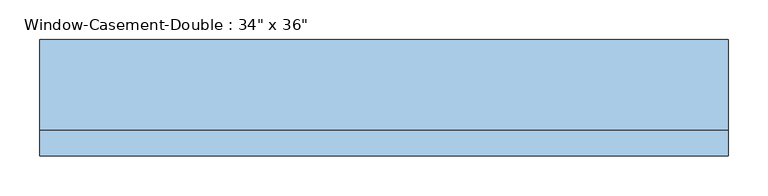
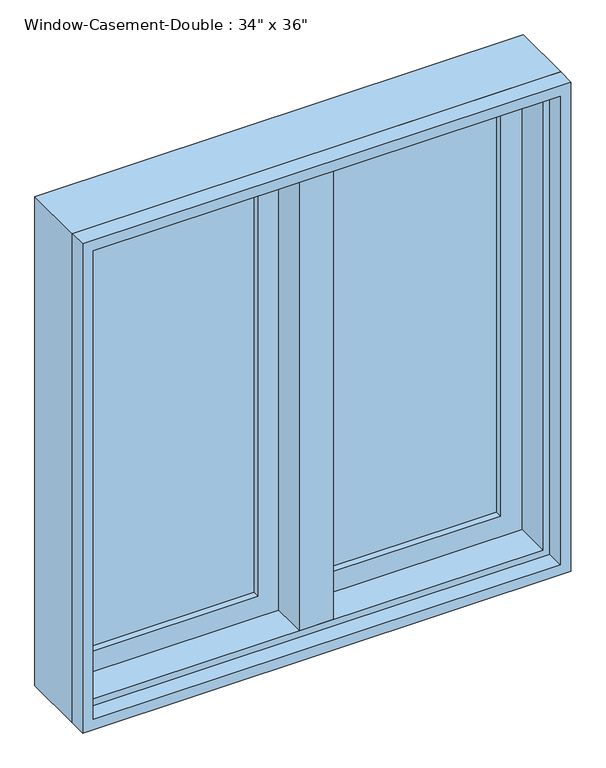
"""IFC4 building model written with IfcOpenShell, lengths in millimetres: window geometry."""

from ifc_helpers import new_model, si_unit, frame, origin, place, context, project, spatial, polyline, outline, extrude, faceted_brep, source, transform, mapped, element, save


def window_0d9958e7(model_context):
    return source(origin(), model_context, "Body", "SolidModel", [
        faceted_brep([(9.525, 82.55, 1816.1), (-9.525, 82.55, 1816.1), (-9.525, 31.75, 1816.1), (9.525, 31.75, 1816.1), (9.525, 82.55, 927.1), (9.525, 31.75, 927.1), (-9.525, 31.75, 927.1), (-9.525, 82.55, 927.1), (-9.525, 31.75, 946.15), (-9.525, 31.75, 1797.05), (-30.1625, 31.75, 946.15), (-30.1625, 31.75, 1797.05), (-30.1625, -31.75, 946.15), (-30.1625, -31.75, 1797.05), (30.1625, -31.75, 946.15), (30.1625, -31.75, 1797.05), (30.1625, 31.75, 946.15), (30.1625, 31.75, 1797.05), (9.525, 31.75, 946.15), (9.525, 31.75, 1797.05)], [[[0, 1, 2, 3]], [[4, 5, 6, 7]], [[1, 0, 4, 7]], [[2, 1, 7, 6, 8, 9]], [[9, 8, 10, 11]], [[11, 10, 12, 13]], [[13, 12, 14, 15]], [[15, 14, 16, 17]], [[17, 16, 18, 19]], [[0, 3, 19, 18, 5, 4]], [[18, 8, 6, 5]], [[9, 19, 3, 2]], [[8, 18, 16, 14, 12, 10]], [[19, 9, 11, 13, 15, 17]]]),
        extrude(outline(polyline([(-66.675, 63.5), (-66.675, 57.15), (-361.95, 57.15), (-361.95, 63.5), (-66.675, 63.5)])), frame((0.0, 0.0, 984.25), z_axis=(0.0, 0.0, 1.0), x_axis=(1.0, 0.0, 0.0)), (0.0, 0.0, 1.0), 774.7),
        extrude(outline(polyline([(-361.95, 44.45), (-361.95, 50.8), (-66.675, 50.8), (-66.675, 44.45), (-361.95, 44.45)])), frame((0.0, 0.0, 984.25), z_axis=(0.0, 0.0, 1.0), x_axis=(1.0, 0.0, 0.0)), (0.0, 0.0, 1.0), 774.7),
        extrude(outline(polyline([(361.95, 63.5), (361.95, 57.15), (66.675, 57.15), (66.675, 63.5), (361.95, 63.5)])), frame((0.0, 0.0, 984.25), z_axis=(0.0, 0.0, 1.0), x_axis=(1.0, 0.0, 0.0)), (0.0, 0.0, 1.0), 774.7),
        extrude(outline(polyline([(66.675, 44.45), (66.675, 50.8), (361.95, 50.8), (361.95, 44.45), (66.675, 44.45)])), frame((0.0, 0.0, 984.25), z_axis=(0.0, 0.0, 1.0), x_axis=(1.0, 0.0, 0.0)), (0.0, 0.0, 1.0), 774.7),
        extrude(outline(polyline([(1816.1, -419.1), (927.1, -419.1), (927.1, -9.525), (1816.1, -9.525), (1816.1, -419.1)]), holes=[polyline([(1758.95, -66.675), (984.25, -66.675), (984.25, -361.95), (1758.95, -361.95), (1758.95, -66.675)])]), frame((0.0, 31.75, 0.0), z_axis=(0.0, 1.0, 0.0), x_axis=(0.0, 0.0, 1.0)), (0.0, 0.0, 1.0), 44.45),
        extrude(outline(polyline([(927.1, 419.1), (1816.1, 419.1), (1816.1, 9.525), (927.1, 9.525), (927.1, 419.1)]), holes=[polyline([(984.25, 66.675), (1758.95, 66.675), (1758.95, 361.95), (984.25, 361.95), (984.25, 66.675)])]), frame((0.0, 31.75, 0.0), z_axis=(0.0, 1.0, 0.0), x_axis=(0.0, 0.0, 1.0)), (0.0, 0.0, 1.0), 44.45),
        extrude(outline(polyline([(1828.8, -431.8), (914.4, -431.8), (914.4, 431.8), (1828.8, 431.8), (1828.8, -431.8)]), holes=[polyline([(1809.75, 412.75), (933.45, 412.75), (933.45, -412.75), (1809.75, -412.75), (1809.75, 412.75)])]), frame((0.0, -63.5, 0.0), z_axis=(0.0, 1.0, 0.0), x_axis=(0.0, 0.0, 1.0)), (0.0, 0.0, 1.0), 31.75),
        faceted_brep([(400.05, 31.75, 1797.05), (400.05, -31.75, 1797.05), (-400.05, -31.75, 1797.05), (-400.05, 31.75, 1797.05), (419.1, 82.55, 1816.1), (419.1, 31.75, 1816.1), (-419.1, 31.75, 1816.1), (-419.1, 82.55, 1816.1), (431.8, -31.75, 1828.8), (431.8, 82.55, 1828.8), (-431.8, 82.55, 1828.8), (-431.8, -31.75, 1828.8), (-400.05, -31.75, 946.15), (-400.05, 31.75, 946.15), (-419.1, 31.75, 927.1), (-419.1, 82.55, 927.1), (-431.8, 82.55, 914.4), (-431.8, -31.75, 914.4), (400.05, -31.75, 946.15), (400.05, 31.75, 946.15), (419.1, 31.75, 927.1), (419.1, 82.55, 927.1), (431.8, 82.55, 914.4), (431.8, -31.75, 914.4)], [[[0, 1, 2, 3]], [[4, 5, 6, 7]], [[8, 9, 10, 11]], [[3, 2, 12, 13]], [[7, 6, 14, 15]], [[11, 10, 16, 17]], [[13, 12, 18, 19]], [[15, 14, 20, 21]], [[17, 16, 22, 23]], [[11, 17, 23, 8], [1, 18, 12, 2]], [[19, 18, 1, 0]], [[5, 20, 14, 6], [3, 13, 19, 0]], [[21, 20, 5, 4]], [[23, 22, 9, 8]], [[9, 22, 16, 10], [7, 15, 21, 4]]]),
    ])


if __name__ == "__main__":
    model = new_model("IFC4")
    model_context = context("Model", 3, world=origin())
    ifc_project = project(units=[si_unit("LENGTHUNIT", "METRE", prefix="MILLI")], contexts=[model_context])
    site = spatial("IfcSite", under=ifc_project)
    building = spatial("IfcBuilding", under=site)
    placement = place(None, origin())
    window_shape = window_0d9958e7(model_context)
    element("IfcWindow", 1, ObjectType="Window-Casement-Double : 34\" x 36\"", at=placement, inside=building, context=model_context, shape_type="MappedRepresentation", body=[
        mapped(window_shape, transform((0.0, 0.0, 0.0), x_axis=(1.0, 0.0, 0.0), y_axis=(0.0, 1.0, 0.0), z_axis=(0.0, 0.0, 1.0))),
    ])
    save(model, "model.ifc")

# Revit data of these elements
# Type "Window-Casement-Double : 34\" x 36\""
#   Type Mark = "14"
#   Fire Rating = "0.5h"
#   Assembly Code = "B2020100"
#   Analytic Construction = "Double glazing - domestic"
#   Frame Extension [instance default] = 0' - 0 1/4"
#   Window Inset [instance default] = 0' - 0"
#   Wall Thickness [instance default] = 0' - 6"
#   Interior Wall Closure [instance default] = 0' - 2 1/4"
#   Half Width = 1' - 5"
#   Visual Light Transmittance = 0.81
#   Thermal Resistance (R) = 1.8146 (h·ft²·°F)/BTU
#   Solar Heat Gain Coefficient = 0.76
#   Rough Width = 2' - 10 1/2"
#   Rough Height = 3' - 0 1/2"
#   Height = 3' - 0"
#   Heat Transfer Coefficient (U) = 0.5511 BTU/(h·ft²·°F)
#   Exterior Wall Closure [instance default] = 0' - 1 1/4"
#   Extension Jamb [instance default] = 0' - 2 1/4"
#   Default Sill Height = 3' - 0"
#   Width = 2' - 10"
#   Define Thermal Properties by = 0
#   Muntin Visibility = yes
#   Interior Trim Visibility [instance default] = yes
#   Exterior Trim Visibility [instance default] = yes
#   Extension Jamb Visibility [instance default] = yes
#   Interior Trim Material = Wood - Stained
#   Muntin Pattern = Muntin Pattern_2x2 : Muntin Pattern_2x2
#   Interior Trim = Trim-Window-Interior-Flat : Picture Frame
#   Interior Frame Material = Wood - Stained
#   Glass Panel Material = Glass
#   Exterior Trim Material = Clad - White
#   Exterior Trim = Trim-Window-Exterior-Flat : with Sill
#   Exterior Frame Material = Clad - White
#   Wall Closure = (empty or 0)
# Element 1 (IfcWindow, "Window-Casement-Double : 34\" x 36\"")
#   Wall Thickness = 0' - 5"
#   Extension Jamb = 0' - 1 1/4"
#   Materials on its faces: "Wood - Stained", "Glass", "Clad - White"
# Materials
#   "Wood - Stained": class "Wood", colour RGB 224 178 126, transparency 0, Cost = 0
#   "Glass": class "Glass", colour RGB 0 128 192, transparency 0.75, Description = "Soda Lime Glass", Cost = 0
#   "Clad - White": class "Wood", colour RGB 242 242 238, transparency 0, Cost = 0
